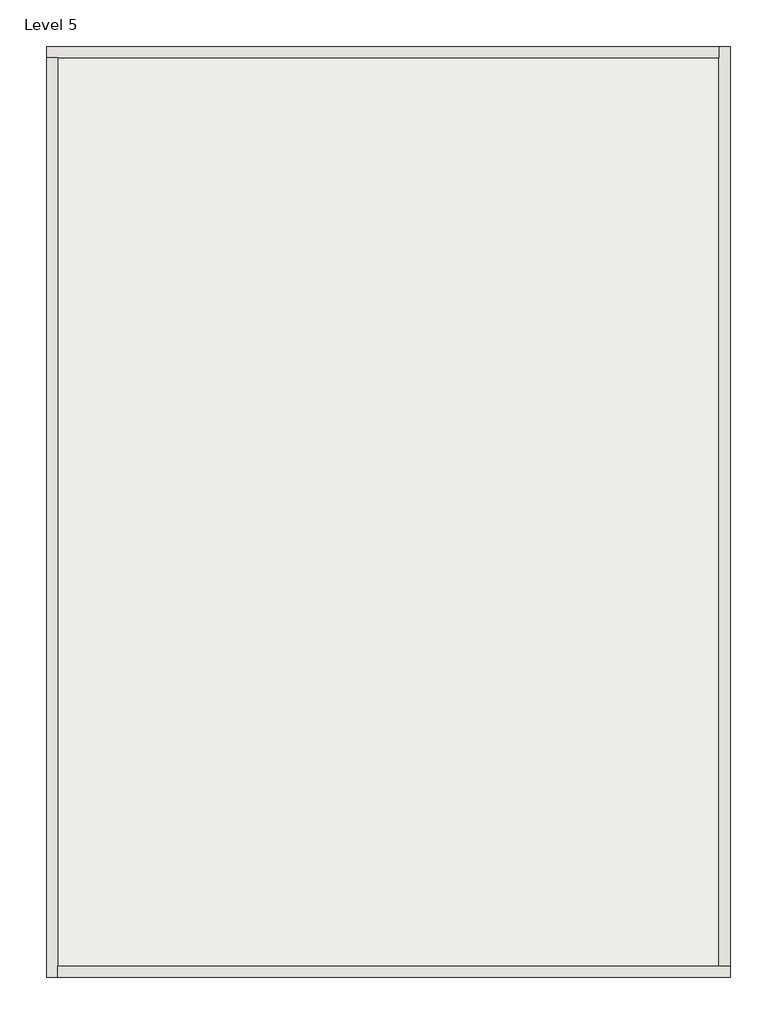
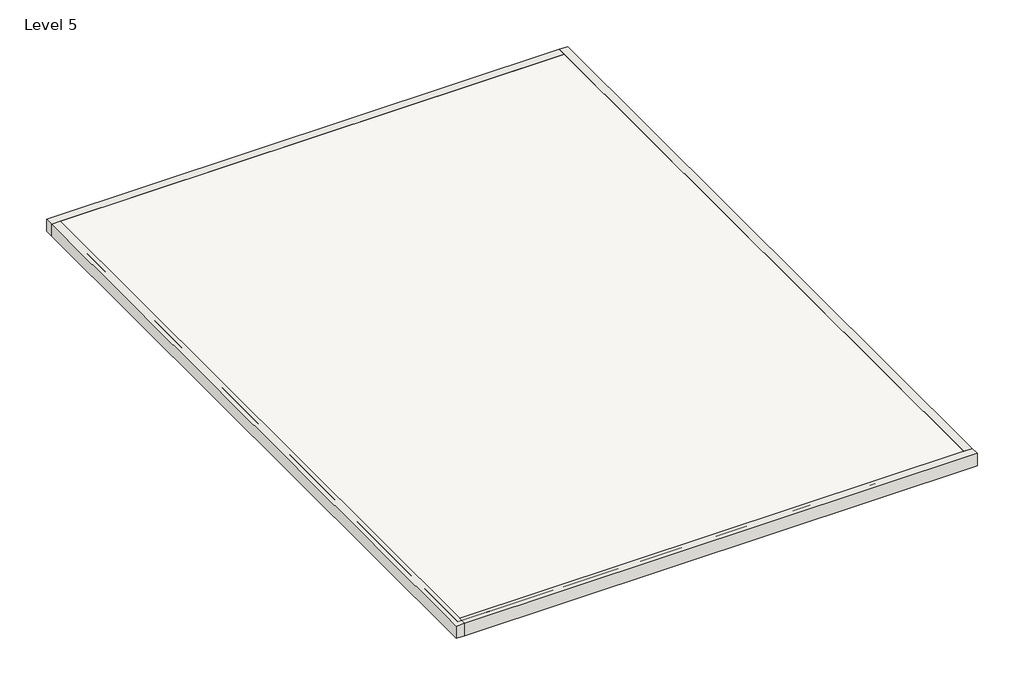
# One storey, incomplete: 4 walls, 1 roof.
"""IFC4 building model written with IfcOpenShell, lengths in millimetres."""

from ifc_helpers import new_model, si_unit, frame, origin, place, context, project, spatial, polyline, outline, extrude, faceted_brep, element, save

model = new_model("IFC4")

# Units and contexts
model_context = context("Model", 3, world=origin())
ifc_project = project(units=[si_unit("LENGTHUNIT", "METRE", prefix="MILLI")], contexts=[model_context])

# Site, building, storey
site = spatial("IfcSite", under=ifc_project)
building = spatial("IfcBuilding", under=site)
storey = spatial("IfcBuildingStorey", under=building, Name="Level 5", Elevation=12192.0)

# Roof
placement = place(None, origin())
element("IfcRoof", 1, ObjectType="Generic - 12\"", at=placement, inside=storey, context=model_context, shape_type="SweptSolid", body=[
    extrude(outline(polyline([(-7048.0058717, 8321.6547293), (5029.6941283, 8321.6547293), (5029.6941283, -8124.8452707), (-7048.0058717, -8124.8452707), (-7048.0058717, 8321.6547293)])), frame((0.0, 0.0, 12192.0), z_axis=(0.0, 0.0, 1.0), x_axis=(1.0, 0.0, 0.0)), (0.0, 0.0, 1.0), 304.8),
])

# Walls
element("IfcWall", 2, ObjectType="Generic - 9\"", at=placement, inside=storey, context=model_context, shape_type="Brep", body=[
    faceted_brep([(-7149.6058717, 8220.0547293, 12192.0), (-6946.4058717, 8220.0547293, 12192.0), (4889.9941283, 8220.0547293, 12192.0), (4889.9941283, 8220.0547293, 12496.8), (-6946.4058717, 8220.0547293, 12496.8), (-7149.6058717, 8220.0547293, 12496.8), (-7149.6058717, 8423.2547293, 12192.0), (-7149.6058717, 8423.2547293, 12496.8), (4889.9941283, 8423.2547293, 12496.8), (4889.9941283, 8423.2547293, 12192.0)], [[[0, 1, 2, 3, 4, 5]], [[6, 7, 8, 9]], [[2, 1, 0, 6, 9]], [[5, 4, 3, 8, 7]], [[0, 5, 7, 6]], [[3, 2, 9, 8]]]),
])
element("IfcWall", 3, ObjectType="Generic - 9\"", at=placement, inside=storey, context=model_context, shape_type="Brep", body=[
    faceted_brep([(-6946.4058717, -8239.1452707, 12192.0), (-6946.4058717, -8035.9452707, 12192.0), (-6946.4058717, 8220.0547293, 12192.0), (-6946.4058717, 8220.0547293, 12496.8), (-6946.4058717, -8035.9452707, 12496.8), (-6946.4058717, -8239.1452707, 12496.8), (-7149.6058717, -8239.1452707, 12192.0), (-7149.6058717, -8239.1452707, 12496.8), (-7149.6058717, 8220.0547293, 12496.8), (-7149.6058717, 8220.0547293, 12192.0)], [[[0, 1, 2, 3, 4, 5]], [[6, 7, 8, 9]], [[2, 1, 0, 6, 9]], [[5, 4, 3, 8, 7]], [[0, 5, 7, 6]], [[3, 2, 9, 8]]]),
])
element("IfcWall", 4, ObjectType="Generic - 9\"", at=placement, inside=storey, context=model_context, shape_type="Brep", body=[
    faceted_brep([(5093.1941283, -8035.9452707, 12192.0), (4889.9941283, -8035.9452707, 12192.0), (-6946.4058717, -8035.9452707, 12192.0), (-6946.4058717, -8035.9452707, 12496.8), (4889.9941283, -8035.9452707, 12496.8), (5093.1941283, -8035.9452707, 12496.8), (5093.1941283, -8239.1452707, 12192.0), (5093.1941283, -8239.1452707, 12496.8), (-6946.4058717, -8239.1452707, 12496.8), (-6946.4058717, -8239.1452707, 12192.0)], [[[0, 1, 2, 3, 4, 5]], [[6, 7, 8, 9]], [[2, 1, 0, 6, 9]], [[5, 4, 3, 8, 7]], [[0, 5, 7, 6]], [[3, 2, 9, 8]]]),
])
element("IfcWall", 5, ObjectType="Generic - 9\"", at=placement, inside=storey, context=model_context, shape_type="Brep", body=[
    faceted_brep([(4889.9941283, 8423.2547293, 12192.0), (4889.9941283, 8220.0547293, 12192.0), (4889.9941283, -8035.9452707, 12192.0), (4889.9941283, -8035.9452707, 12496.8), (4889.9941283, 8220.0547293, 12496.8), (4889.9941283, 8423.2547293, 12496.8), (5093.1941283, 8423.2547293, 12192.0), (5093.1941283, 8423.2547293, 12496.8), (5093.1941283, -8035.9452707, 12496.8), (5093.1941283, -8035.9452707, 12192.0)], [[[0, 1, 2, 3, 4, 5]], [[6, 7, 8, 9]], [[2, 1, 0, 6, 9]], [[5, 4, 3, 8, 7]], [[0, 5, 7, 6]], [[3, 2, 9, 8]]]),
])

save(model, "model.ifc")

# Revit data of these elements
# Type "Generic - 12\""
#   Assembly Code = "B1020"
#   Layers, outside or top first: 1' - 0" no material (function 1)
# Type "Generic - 9\""
#   Assembly Code = "B2010"
#   Layers, outside or top first: 0' - 8" no material (function 1)
# Element 1 (IfcRoof, "Generic - 12\"")
#   built-in parameter 1001705 = 41 (stored number, unit not read)
#   built-in parameter 1001710 = 33615
#   Phase Created = New Construction
#   Materials on its faces: "Default Roof"
# Element 2 (IfcWall, "Generic - 9\"")
#   Top Offset = 0' - 0"
#   Base Offset = 0' - 0"
#   Unconnected Height = 1' - 0"
#   wall height = 1' - 0"
#   Phase Created = New Construction
#   Base Constraint = Level 5
#   Materials on its faces: "Default Wall", "Brick, Soldier Course"
# Element 3 (IfcWall, "Generic - 9\"")
#   Top Offset = 0' - 0"
#   Base Offset = 0' - 0"
#   Unconnected Height = 1' - 0"
#   wall height = 1' - 0"
#   Phase Created = New Construction
#   Base Constraint = Level 5
#   Materials on its faces: "Default Wall", "Brick, Soldier Course", "Parking Stripe"
# Element 4 (IfcWall, "Generic - 9\"")
#   Top Offset = 0' - 0"
#   Base Offset = 0' - 0"
#   Unconnected Height = 1' - 0"
#   wall height = 1' - 0"
#   Phase Created = New Construction
#   Base Constraint = Level 5
#   Materials on its faces: "Default Wall", "Parking Stripe", "Door - Frame/Mullion"
# Element 5 (IfcWall, "Generic - 9\"")
#   Top Offset = 0' - 0"
#   Base Offset = 0' - 0"
#   Unconnected Height = 1' - 0"
#   wall height = 1' - 0"
#   Phase Created = New Construction
#   Base Constraint = Level 5
#   Materials on its faces: "Default Wall", "Door - Frame/Mullion"
# Materials
#   "Default Roof": colour RGB 88 101 114, transparency 0, Cost = 0
#   "Default Wall": colour RGB 128 128 128, transparency 0, Cost = 0
#   "Brick, Soldier Course": class "Masonry", colour RGB 170 98 104, transparency 0, Description = "Common brick soldier coursed", Cost = 0
#   "Parking Stripe": class "Paint", colour RGB 250 250 91, transparency 0, Cost = 0
#   "Door - Frame/Mullion": class "Wood", colour RGB 212 179 113, transparency 0
